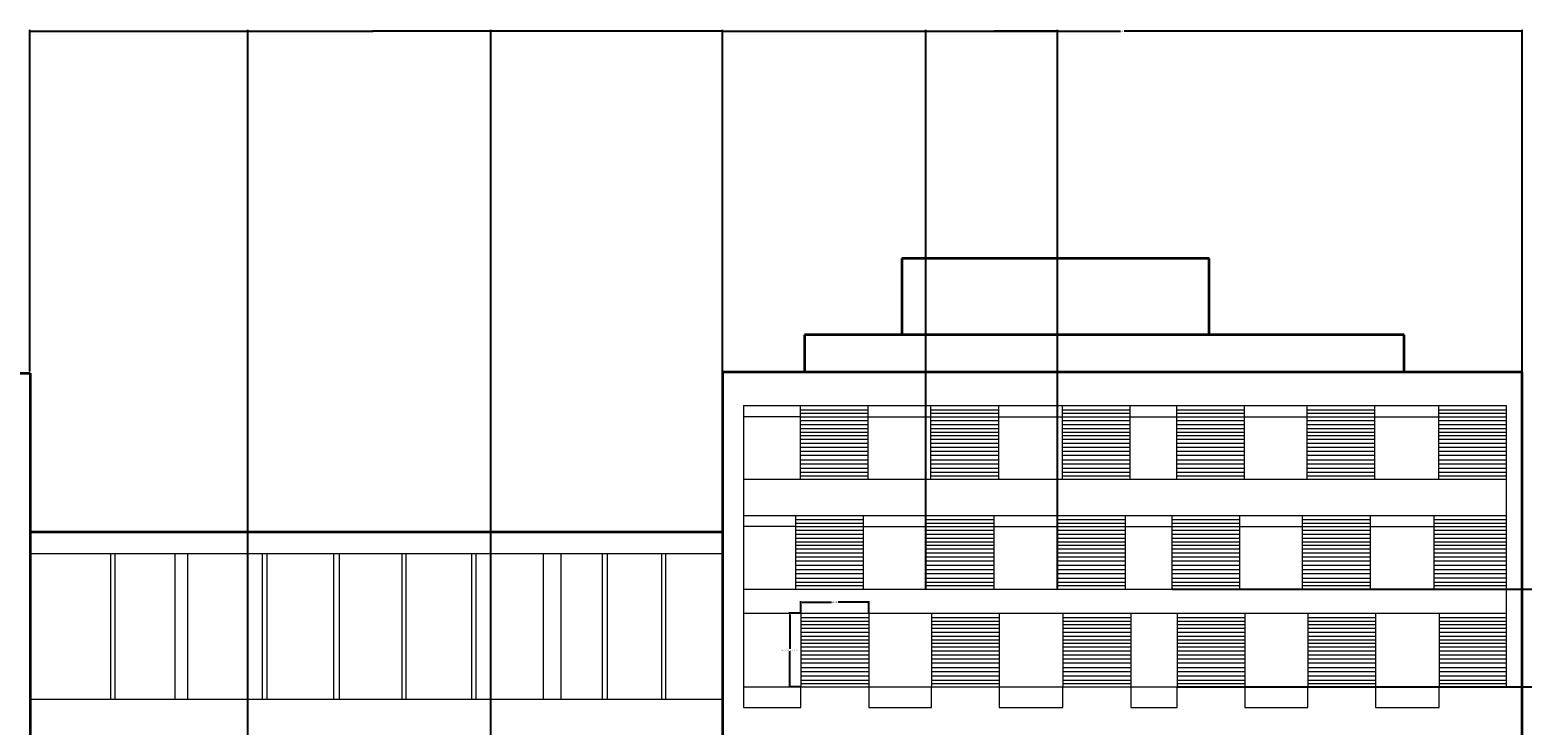
# Model space of a CAD drawing. Units: inches. Extents: x -279 to 364, y -385 to 335.
# Tile 3 of 9: x 7 to 238, y -185 to -78. Entities that reach past the tile are written whole.
import ezdxf

# ---------------------------------------------------------------- set-up
doc = ezdxf.new("R2010")
doc.units = ezdxf.units.IN
doc.header["$MEASUREMENT"] = 0
for name, color, linetype, lineweight in [('A-ANNO-DIMS', 2, 'Continuous', 18), ('A-GLAZ-CURT', 4, 'Continuous', 18), ('A-ROOF', 7, 'Continuous', 35), ('A-WALL', 7, 'Continuous', 35), ('A-WALL-LOUV', 8, 'Continuous', 13)]:
    doc.layers.add(name, color=color, linetype=linetype, lineweight=lineweight)
doc.styles.get("Standard").update_dxf_attribs({"font": 'arial.ttf'})
doc.dimstyles.get("Standard").update_dxf_attribs({"dimtxt": 0.18, "dimasz": 0.18, "dimexe": 0.18, "dimexo": 0.0625, "dimgap": 0.09, "dimtad": 0, "dimtih": 1, "dimtoh": 1, "dimdec": 4, "dimzin": 0, "dimdsep": 46, "dimtxsty": 'Standard', "dimcen": 0.09, "dimadec": 0, "dimazin": 0, "dimtfac": 1, "dimtdec": 4, "dimtofl": 0, "dimtmove": 0, "dimatfit": 3, "dimfxl": 1, "dimtolj": 1, "dimtzin": 0, "dimarcsym": 0})

# ---------------------------------------------------------------- blocks, each defined once
blk = doc.blocks.new('LOUVER-SIDE-UPPER')
for p, q in [((0, 11.42), (10.51, 11.42)), ((0, 11.42), (0, 0)), ((0, 10.78), (10.51, 10.78)), ((0, 10.22), (10.51, 10.22)), ((0, 9.68), (10.51, 9.68)), ((10.51, 11.42), (10.51, 0)), ((0, 9.11), (10.51, 9.11)), ((0, 8.49), (10.51, 8.49)), ((0, 7.88), (10.51, 7.88)), ((0, 7.3), (10.51, 7.3)), ((0, 6.79), (10.51, 6.79)), ((0, 6.22), (10.51, 6.22)), ((0, 5.6), (10.51, 5.6)), ((0, 4.97), (10.51, 4.97)), ((0, 4.37), (10.51, 4.37)), ((0, 3.72), (10.51, 3.72)), ((0, 3.01), (10.51, 3.01)), ((0, 2.4), (10.51, 2.4)), ((0, 1.71), (10.51, 1.71)), ((0, 1.07), (10.51, 1.07)), ((0, 0.54), (10.51, 0.54))]:
    blk.add_line(p, q)
blk = doc.blocks.new('*D46')
at = {"layer": 'A-ANNO-DIMS', "color": 0, "lineweight": -2, "transparency": 16777216}
for p, q in [((126.46, -168.11), (124.63, -168.11)), ((124.81, -168.29), (124.81, -173.64)), ((124.81, -179.35), (124.81, -174)), ((126.46, -179.53), (124.63, -179.53))]:
    blk.add_line(p, q, dxfattribs=at)
at = {"layer": 'A-ANNO-DIMS', "color": 0, "transparency": 16777216}
for points in [[(124.78, -168.29), (124.84, -168.29), (124.81, -168.11)], [(124.78, -179.35), (124.84, -179.35), (124.81, -179.53)]]:
    blk.add_solid(points, dxfattribs=at)
at = {"layer": 'Defpoints', "color": 0, "transparency": 16777216}
for p in [(124.81, -168.11), (126.52, -168.11), (126.52, -179.53)]:
    blk.add_point(p, dxfattribs=at)
at = {"layer": 'A-ANNO-DIMS', "color": 0, "transparency": 16777216, "insert": (124.81, -173.82), "char_height": 0.18, "attachment_point": 5}
blk.add_mtext('\\A1;UPPER LOUVER 11 TYP.', dxfattribs=at)
blk = doc.blocks.new('*D47')
at = {"layer": 'A-ANNO-DIMS', "color": 0, "lineweight": -2, "transparency": 16777216}
for p, q in [((126.52, -168.05), (126.52, -166.22)), ((126.7, -166.4), (131.25, -166.4)), ((136.85, -166.4), (132.29, -166.4)), ((137.03, -168.05), (137.03, -166.22))]:
    blk.add_line(p, q, dxfattribs=at)
at = {"layer": 'A-ANNO-DIMS', "color": 0, "transparency": 16777216}
for points in [[(126.7, -166.37), (126.7, -166.43), (126.52, -166.4)], [(136.85, -166.37), (136.85, -166.43), (137.03, -166.4)]]:
    blk.add_solid(points, dxfattribs=at)
at = {"layer": 'Defpoints', "color": 0, "transparency": 16777216}
for p in [(137.03, -166.4), (126.52, -168.11), (137.03, -168.11)]:
    blk.add_point(p, dxfattribs=at)
at = {"layer": 'A-ANNO-DIMS', "color": 0, "transparency": 16777216, "insert": (131.77, -166.4), "char_height": 0.18, "attachment_point": 5}
blk.add_mtext('\\A1;11 TYP.', dxfattribs=at)
blk = doc.blocks.new('*D100')
at = {"layer": 'A-ANNO-DIMS', "color": 0, "lineweight": -2, "transparency": 16777216}
for p, q in [((6.96, -130.63), (6.96, -77.65)), ((7.14, -77.83), (60.2, -77.83)), ((114.17, -77.83), (61.11, -77.83)), ((114.35, -130.65), (114.35, -77.65))]:
    blk.add_line(p, q, dxfattribs=at)
at = {"layer": 'A-ANNO-DIMS', "color": 0, "transparency": 16777216}
for points in [[(7.14, -77.8), (7.14, -77.86), (6.96, -77.83)], [(114.17, -77.8), (114.17, -77.86), (114.35, -77.83)]]:
    blk.add_solid(points, dxfattribs=at)
at = {"layer": 'Defpoints', "color": 0, "transparency": 16777216}
for p in [(114.35, -77.83), (6.96, -130.69), (114.35, -130.71)]:
    blk.add_point(p, dxfattribs=at)
at = {"layer": 'A-ANNO-DIMS', "color": 0, "transparency": 16777216, "insert": (60.65, -77.83), "char_height": 0.18, "attachment_point": 5}
blk.add_mtext('\\A1;107.38', dxfattribs=at)
blk = doc.blocks.new('*D101')
at = {"layer": 'A-ANNO-DIMS', "color": 0, "lineweight": -2, "transparency": 16777216}
for p, q in [((114.35, -130.65), (114.35, -77.65)), ((114.53, -77.83), (176.06, -77.83)), ((238.16, -77.83), (176.62, -77.83)), ((238.34, -130.65), (238.34, -77.65))]:
    blk.add_line(p, q, dxfattribs=at)
at = {"layer": 'A-ANNO-DIMS', "color": 0, "transparency": 16777216}
for points in [[(114.53, -77.8), (114.53, -77.86), (114.35, -77.83)], [(238.16, -77.8), (238.16, -77.86), (238.34, -77.83)]]:
    blk.add_solid(points, dxfattribs=at)
at = {"layer": 'Defpoints', "color": 0, "transparency": 16777216}
for p in [(238.34, -77.83), (114.35, -130.71), (238.34, -130.71)]:
    blk.add_point(p, dxfattribs=at)
at = {"layer": 'A-ANNO-DIMS', "color": 0, "transparency": 16777216, "insert": (176.34, -77.83), "char_height": 0.18, "attachment_point": 5}
blk.add_mtext('\\A1;124', dxfattribs=at)
blk = doc.blocks.new('*D110')
at = {"layer": 'A-ANNO-DIMS', "color": 0, "lineweight": -2, "transparency": 16777216}
for p, q in [((145.91, -164.29), (145.91, -77.65)), ((146.09, -77.83), (155.71, -77.83)), ((166.12, -77.83), (156.5, -77.83)), ((166.3, -164.29), (166.3, -77.65))]:
    blk.add_line(p, q, dxfattribs=at)
at = {"layer": 'A-ANNO-DIMS', "color": 0, "transparency": 16777216}
for points in [[(146.09, -77.8), (146.09, -77.86), (145.91, -77.83)], [(166.12, -77.8), (166.12, -77.86), (166.3, -77.83)]]:
    blk.add_solid(points, dxfattribs=at)
at = {"layer": 'Defpoints', "color": 0, "transparency": 16777216}
for p in [(166.3, -77.83), (145.91, -164.35), (166.3, -164.35)]:
    blk.add_point(p, dxfattribs=at)
at = {"layer": 'A-ANNO-DIMS', "color": 0, "transparency": 16777216, "insert": (156.11, -77.83), "char_height": 0.18, "attachment_point": 5}
blk.add_mtext('\\A1;20.39', dxfattribs=at)
blk = doc.blocks.new('*D111')
at = {"layer": 'A-ANNO-DIMS', "color": 0, "lineweight": -2, "transparency": 16777216}
for p, q in [((184.08, -164.35), (361.74, -164.35)), ((361.56, -164.53), (361.56, -171.76)), ((361.56, -179.35), (361.56, -172.12)), ((184.92, -179.53), (361.74, -179.53))]:
    blk.add_line(p, q, dxfattribs=at)
at = {"layer": 'A-ANNO-DIMS', "color": 0, "transparency": 16777216}
for points in [[(361.53, -164.53), (361.59, -164.53), (361.56, -164.35)], [(361.53, -179.35), (361.59, -179.35), (361.56, -179.53)]]:
    blk.add_solid(points, dxfattribs=at)
at = {"layer": 'Defpoints', "color": 0, "transparency": 16777216}
for p in [(184.01, -164.35), (184.86, -179.53), (361.56, -179.53)]:
    blk.add_point(p, dxfattribs=at)
at = {"layer": 'A-ANNO-DIMS', "color": 0, "transparency": 16777216, "insert": (361.56, -171.94), "char_height": 0.18, "attachment_point": 5}
blk.add_mtext('\\A1;15.182', dxfattribs=at)
blk = doc.blocks.new('*D115')
at = {"layer": 'A-ANNO-DIMS', "color": 0, "lineweight": -2, "transparency": 16777216}
for p, q in [((40.79, -273.55), (40.79, -77.65)), ((40.97, -77.83), (59.16, -77.83)), ((78.28, -77.83), (60.09, -77.83)), ((78.46, -273.55), (78.46, -77.65))]:
    blk.add_line(p, q, dxfattribs=at)
at = {"layer": 'A-ANNO-DIMS', "color": 0, "transparency": 16777216}
for points in [[(40.97, -77.8), (40.97, -77.86), (40.79, -77.83)], [(78.28, -77.8), (78.28, -77.86), (78.46, -77.83)]]:
    blk.add_solid(points, dxfattribs=at)
at = {"layer": 'Defpoints', "color": 0, "transparency": 16777216}
for p in [(78.46, -77.83), (40.79, -273.62), (78.46, -273.62)]:
    blk.add_point(p, dxfattribs=at)
at = {"layer": 'A-ANNO-DIMS', "color": 0, "transparency": 16777216, "insert": (59.62, -77.83), "char_height": 0.18, "attachment_point": 5}
blk.add_mtext('\\A1;37.665', dxfattribs=at)

msp = doc.modelspace()

# ---------------------------------------------------------------- linework, layer by layer
at = {"layer": 'A-GLAZ-CURT'}
for p, q in [((7.0091, -158.8588), (114.3455, -158.8588)), ((19.4866, -158.8588), (19.4866, -181.4362)), ((20.1452, -158.8588), (20.1452, -181.4362)), ((29.5321, -181.4362), (29.5321, -158.8588)), ((31.4736, -181.4362), (31.4736, -158.8588)), ((42.982, -158.8588), (42.982, -181.4362)), ((43.738, -158.8588), (43.738, -181.4362)), ((54.0458, -158.8588), (54.0458, -181.4362)), ((54.9191, -158.8588), (54.9191, -181.4362)), ((64.6388, -158.8588), (64.6388, -181.4362)), ((65.2914, -158.8588), (65.2914, -181.4362)), ((75.4672, -158.8588), (75.4672, -181.4362)), ((76.1493, -158.8588), (76.1493, -181.4362)), ((86.6113, -181.4362), (86.6113, -158.8588)), ((89.3294, -181.4362), (89.3294, -158.8588)), ((95.7116, -158.8588), (95.7116, -181.4362)), ((96.4877, -158.8588), (96.4877, -181.4362)), ((104.8922, -158.8588), (104.8922, -181.4362)), ((105.5503, -158.8588), (105.5503, -181.4362)), ((7.0091, -181.4362), (114.3455, -181.4362))]:
    msp.add_line(p, q, dxfattribs=at)
at = {"layer": 'A-ROOF'}
for p, q in [((189.8032, -113.1006), (142.1799, -113.1006)), ((142.1799, -113.1006), (142.1799, -124.9219)), ((189.8032, -124.9219), (189.8032, -113.1006)), ((220.0549, -124.9219), (127.1002, -124.9219)), ((127.1002, -124.9219), (127.1002, -130.7132)), ((220.0549, -130.7132), (220.0549, -124.9219)), ((7.0091, -155.488), (114.3455, -155.488))]:
    msp.add_line(p, q, dxfattribs=at)
at = {"layer": 'A-WALL'}
for p, q in [((-116.9812, -130.861), (7.0091, -130.861)), ((7.0091, -130.861), (7.0091, -188.3649)), ((238.3359, -130.7132), (114.3455, -130.7132)), ((114.3455, -130.7132), (114.3455, -188.2171)), ((238.3359, -188.2171), (238.3359, -130.7132))]:
    msp.add_line(p, q, dxfattribs=at)
at = {"layer": 'A-WALL-LOUV'}
for p, q in [((117.6325, -135.9028), (181.1097, -135.9028)), ((117.6325, -135.9028), (117.6325, -170.5098)), ((181.1097, -135.9028), (235.8547, -135.9028)), ((126.3888, -137.642), (117.6325, -137.642)), ((136.8946, -137.642), (235.8547, -137.642)), ((117.6325, -147.3245), (181.1097, -147.3245)), ((181.1097, -147.3245), (235.8547, -147.3245)), ((235.8547, -147.3245), (235.8547, -168.3948)), ((117.6325, -152.9294), (180.3975, -152.9294)), ((125.6766, -154.6687), (117.6325, -154.6687)), ((136.1824, -154.6687), (235.8547, -154.6687)), ((174.083, -152.9294), (235.1425, -152.9294)), ((224.6367, -152.9294), (224.6367, -164.3511)), ((224.6367, -152.9294), (235.8547, -152.9294)), ((224.6367, -153.5661), (235.8547, -153.5661)), ((224.6367, -154.1327), (235.8547, -154.1327)), ((224.6367, -154.6687), (235.8547, -154.6687)), ((224.6367, -155.2448), (235.8547, -155.2448)), ((224.6367, -155.8634), (235.8547, -155.8634)), ((224.6367, -156.4664), (235.8547, -156.4664)), ((224.6367, -157.056), (235.8547, -157.056)), ((224.6367, -157.5651), (235.8547, -157.5651)), ((224.6367, -158.1319), (235.8547, -158.1319)), ((224.6367, -158.7505), (235.8547, -158.7505)), ((224.6367, -159.3803), (235.8547, -159.3803)), ((224.6367, -159.9833), (235.8547, -159.9833)), ((224.6367, -160.6264), (235.8547, -160.6264)), ((224.6367, -161.3366), (235.8547, -161.3366)), ((224.6367, -161.9558), (235.8547, -161.9558)), ((224.6367, -162.6391), (235.8547, -162.6391)), ((224.6367, -163.2853), (235.8547, -163.2853)), ((224.6367, -163.8079), (235.8547, -163.8079)), ((117.6325, -164.3511), (180.3975, -164.3511)), ((174.083, -164.3511), (235.8547, -164.3511)), ((117.6325, -168.111), (181.2419, -168.111)), ((174.9274, -168.111), (235.8547, -168.111)), ((225.4811, -168.111), (225.4811, -179.5326)), ((225.4811, -168.111), (235.8547, -168.111)), ((225.4811, -168.7477), (235.8547, -168.7477)), ((235.8547, -168.3948), (235.8547, -179.5326)), ((117.6325, -170.5098), (117.6325, -179.5326)), ((225.4811, -169.3142), (235.8547, -169.3142)), ((225.4811, -169.8502), (235.8547, -169.8502)), ((225.4811, -170.4264), (235.8547, -170.4264)), ((225.4811, -171.045), (235.8547, -171.045)), ((225.4811, -171.6479), (235.8547, -171.6479)), ((225.4811, -172.2375), (235.8547, -172.2375)), ((225.4811, -172.7467), (235.8547, -172.7467)), ((225.4811, -173.3134), (235.8547, -173.3134)), ((225.4811, -173.9321), (235.8547, -173.9321)), ((225.4811, -174.5618), (235.8547, -174.5618)), ((225.4811, -175.1648), (235.8547, -175.1648)), ((225.4811, -175.808), (235.8547, -175.808)), ((225.4811, -176.5181), (235.8547, -176.5181)), ((225.4811, -177.1373), (235.8547, -177.1373)), ((225.4811, -177.8207), (235.8547, -177.8207)), ((117.6325, -179.5326), (181.2419, -179.5326)), ((117.6325, -179.5326), (117.6325, -182.696)), ((126.521, -182.696), (126.521, -179.5326)), ((137.0268, -179.5326), (137.0268, -182.696)), ((146.7551, -182.696), (146.7551, -179.5326)), ((157.2609, -179.5326), (157.2609, -182.696)), ((167.1447, -182.696), (167.1447, -179.5326)), ((174.9274, -179.5326), (235.8547, -179.5326)), ((177.6505, -179.5326), (177.6505, -182.696)), ((184.8574, -182.696), (184.8574, -179.5326)), ((195.3632, -179.5326), (195.3632, -182.696)), ((205.0916, -182.696), (205.0916, -179.5326)), ((215.5974, -179.5326), (215.5974, -182.696)), ((225.4811, -178.4668), (235.8547, -178.4668)), ((225.4811, -178.9894), (235.8547, -178.9894)), ((225.4811, -182.696), (225.4811, -179.5326)), ((117.6325, -182.696), (126.521, -182.696)), ((137.0268, -182.696), (146.7551, -182.696)), ((157.2609, -182.696), (167.1447, -182.696)), ((177.6505, -182.696), (184.8574, -182.696)), ((195.3632, -182.696), (205.0916, -182.696)), ((215.5974, -182.696), (225.4811, -182.696))]:
    msp.add_line(p, q, dxfattribs=at)

# ---------------------------------------------------------------- block references
for p in [(126.3892, -147.3244), (146.6234, -147.3244), (167.0129, -147.3244), (184.7256, -147.3244), (204.9598, -147.3244), (225.3493, -147.3244), (125.677, -164.351), (145.9111, -164.351), (166.3007, -164.351), (184.0134, -164.351), (204.2476, -164.351), (126.5214, -179.5325), (146.7556, -179.5325), (167.1451, -179.5325), (184.8578, -179.5325), (205.092, -179.5325)]:
    msp.add_blockref('LOUVER-SIDE-UPPER', p, dxfattribs=at)

# ---------------------------------------------------------------- dimensions: what is measured, and where the dimension line sits
at = {"layer": 'A-ANNO-DIMS'}
for base, p1, p2, override, picture, middle in [((114.3455, -77.8255), (6.9609, -130.6925), (114.3455, -130.7132), {"dimdec": 2, "dimlfac": 1, "dimrnd": 0, "dimzin": 0, "dimdsep": 46, "dimlunit": 2}, '*D100', (60.6532, -77.8255)), ((78.4572, -77.8255), (40.7926, -273.6155), (78.4572, -273.6155), {"dimdec": 3, "dimlfac": 1, "dimrnd": 0, "dimzin": 0, "dimdsep": 46, "dimlunit": 2}, '*D115', (59.6249, -77.8255)), ((238.3359, -77.8255), (114.3455, -130.7132), (238.3359, -130.7132), {"dimdec": 0, "dimlfac": 1, "dimrnd": 0, "dimzin": 0, "dimdsep": 46, "dimlunit": 2}, '*D101', (176.3407, -77.8255)), ((166.3003, -77.8255), (145.9107, -164.3511), (166.3003, -164.3511), {"dimdec": 2, "dimlfac": 1, "dimrnd": 0, "dimzin": 0, "dimdsep": 46, "dimlunit": 2}, '*D110', (156.1055, -77.8255))]:
    dim = msp.add_linear_dim(base=base, p1=p1, p2=p2, dimstyle='Standard', override=override, dxfattribs=at)
    dim.commit()
    dim.dimension.update_dxf_attribs({"geometry": picture, "text_midpoint": middle})
dim = msp.add_linear_dim(base=(137.0268, -166.3977), p1=(126.521, -168.111), p2=(137.0268, -168.111), text='<> TYP.', dimstyle='Standard', override={"dimdec": 0, "dimlfac": 1, "dimrnd": 0, "dimzin": 0, "dimdsep": 46, "dimlunit": 2}, dxfattribs=at)
dim.commit()
dim.dimension.update_dxf_attribs({"geometry": '*D47', "text_midpoint": (131.7739, -166.3977)})
dim = msp.add_linear_dim(base=(361.55885, -179.53263), p1=(184.013, -164.35109), p2=(184.85741, -179.53263), angle=90, dimstyle='Standard', override={"dimdec": 3, "dimlfac": 1, "dimrnd": 0, "dimzin": 0, "dimdsep": 46, "dimlunit": 2}, dxfattribs=at)
dim.commit()
dim.dimension.update_dxf_attribs({"geometry": '*D111', "text_midpoint": (361.55885, -171.94186)})
dim = msp.add_linear_dim(base=(124.8077, -168.111), p1=(126.521, -179.5326), p2=(126.521, -168.111), angle=90, text='UPPER LOUVER <> TYP.', dimstyle='Standard', override={"dimdec": 0, "dimlfac": 1, "dimrnd": 0, "dimzin": 0, "dimdsep": 46, "dimlunit": 2}, dxfattribs=at)
dim.commit()
dim.dimension.update_dxf_attribs({"geometry": '*D46', "text_midpoint": (124.8077, -173.8218)})

doc.saveas('drawing.dxf')
